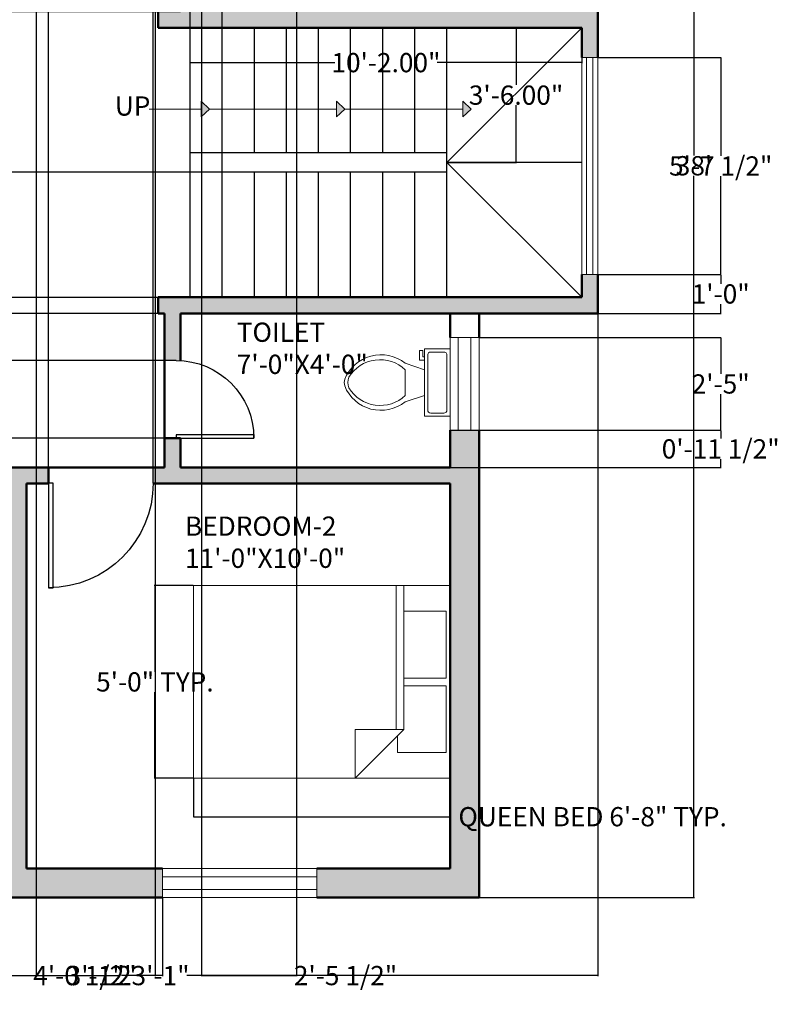
# Model space of a CAD drawing. Units: inches. Extents: x -19 to 356, y -14 to 509.
# Tile 2 of 3: x 118 to 355, y -14 to 293. Entities that reach past the tile are written whole.
import ezdxf

# ---------------------------------------------------------------- set-up
doc = ezdxf.new("R2010")
doc.units = ezdxf.units.IN
doc.header["$MEASUREMENT"] = 0
for name, color, linetype, lineweight in [('A-ANNO-DIMS', 7, 'Continuous', 18), ('A-ANNO-SYMB', 7, 'Continuous', 18), ('A-ANNO-TEXT', 7, 'Continuous', 18), ('A-AREA-IDEN', 7, 'Continuous', 25), ('A-DOOR', 3, 'Continuous', 25), ('A-FLOR-FIXT', 9, 'Continuous', 18), ('A-FLOR-STRS', 7, 'Continuous', 25), ('A-FURN', 8, 'Continuous', 18), ('A-GLAZ', 5, 'Continuous', 18), ('A-WALL', 7, 'Continuous', 50), ('A-WALL-PATT', 4, 'Continuous', 13)]:
    doc.layers.add(name, color=color, linetype=linetype, lineweight=lineweight)
doc.styles.get("Standard").update_dxf_attribs({"font": 'arial.ttf'})
doc.dimstyles.get("Standard").update_dxf_attribs({"dimtxt": 6, "dimasz": 0.18, "dimexe": 0.18, "dimexo": 0.0625, "dimgap": 0.09, "dimtad": 0, "dimtih": 1, "dimtoh": 1, "dimzin": 0, "dimdsep": 46, "dimlunit": 3, "dimtxsty": 'Standard', "dimcen": 0.09, "dimadec": 0, "dimazin": 0, "dimtfac": 1, "dimtofl": 0, "dimtmove": 0, "dimatfit": 3, "dimfxl": 1, "dimtolj": 1, "dimtzin": 0, "dimarcsym": 0})

# ---------------------------------------------------------------- blocks, each defined once
blk = doc.blocks.new('*U2')
for p, q in [((0, 0), (0, -6)), ((40, 0), (40, -6))]:
    blk.add_line(p, q)
blk.add_lwpolyline([(0, 0), (0, 40), (1.75, 40), (1.75, 0)], close=True)
blk.add_arc((0, 0), 40, 0, 90)
blk = doc.blocks.new('*U4')
for p, q in [((9.5, -6), (9.5, -2)), ((-10, -8.5), (-8, -8.5)), ((-10, -9.5), (-10, -8.5)), ((-8, -8.5), (-8, -8)), ((-7, -8), (-7, -9.5)), ((-4, -8), (-6, -14)), ((4, -8), (6, -14)), ((-7, -9.5), (-10, -9.5)), ((4, -14), (-4, -14))]:
    blk.add_line(p, q)
blk.add_lwpolyline([(10.5, -8), (10.5, 0), (-10.5, 0), (-10.5, -8)], close=True)
for points in [[(-9.5, -2), (-9.5, -6)], [(8.5, -1), (-8.5, -1)], [(-8.5, -7), (8.5, -7)]]:
    blk.add_lwpolyline(points)
for centre, radius, start, end in [((-8.62, -1.88), 0.884, 81.8699, 188.1301), ((8.62, -1.88), 0.884, 351.8699, 98.1301), ((-8.62, -6.12), 0.884, 171.8699, 278.1301), ((8.62, -6.12), 0.884, 261.8699, 8.1301), ((3.52, -21.58), 12.17, 141.4691, 247.9714), ((4.2, -21.82), 11.33, 136.3677, 238.9468), ((-3.52, -21.58), 12.17, 292.0284, 38.5307), ((-4.2, -21.82), 11.33, 301.053, 43.6321), ((0, -27.88), 4, 245.7318, 294.2682), ((0, -29), 4, 254.8605, 285.1395)]:
    blk.add_arc(centre, radius, start, end)
blk = doc.blocks.new('Bed - Queen')
for p, q in [((0, -80.00003), (0, 0)), ((0, 0), (59.99999, 0)), ((59.99999, 0), (59.99999, -80.00003)), ((7.99999, -1.2), (28.79998, -1.2)), ((7.99999, -14.4), (7.99999, -1.2)), ((28.79998, -1.2), (28.79998, -14.4)), ((31.19999, -1.2), (51.99999, -1.2)), ((31.19999, -14.4), (31.19999, -1.2)), ((51.99999, -1.2), (51.99999, -16.4)), ((0, -14.4), (44.8, -14.4)), ((59.99999, -29.6), (44.8, -14.4)), ((44.8, -14.4), (44.8, -29.6)), ((44.8, -16.8), (0, -16.8)), ((51.99999, -16.4), (46.79936, -16.4)), ((44.8, -29.6), (59.99999, -29.6)), ((59.99999, -80.00003), (0, -80.00003))]:
    blk.add_line(p, q)
blk = doc.blocks.new('*D8')
at = {"layer": 'A-ANNO-DIMS', "color": 0, "lineweight": -2, "transparency": 16777216}
for p, q in [((261.66, 475.37), (328.76, 475.37)), ((328.58, 475.19), (328.58, 250.53)), ((328.58, 19.55), (328.58, 244.22)), ((261.66, 19.37), (328.76, 19.37))]:
    blk.add_line(p, q, dxfattribs=at)
at = {"layer": 'A-ANNO-DIMS', "color": 0, "transparency": 16777216}
for points in [[(328.55, 475.19), (328.61, 475.19), (328.58, 475.37)], [(328.55, 19.55), (328.61, 19.55), (328.58, 19.37)]]:
    blk.add_solid(points, dxfattribs=at)
at = {"layer": 'Defpoints', "color": 0, "transparency": 16777216}
for p in [(261.6, 475.37), (328.58, 475.37), (261.6, 19.37)]:
    blk.add_point(p, dxfattribs=at)
at = {"layer": 'A-ANNO-DIMS', "color": 0, "transparency": 16777216, "insert": (328.58, 247.37), "char_height": 6, "attachment_point": 5}
blk.add_mtext("\\A1;38'", dxfattribs=at)
blk = doc.blocks.new('*D10')
at = {"layer": 'A-ANNO-DIMS', "color": 0, "lineweight": -2, "transparency": 16777216}
for p, q in [((171.6, 278.44), (171.6, 279.68)), ((171.78, 279.5), (216.66, 279.5)), ((293.42, 279.5), (248.54, 279.5)), ((293.6, 281.06), (293.6, 279.32))]:
    blk.add_line(p, q, dxfattribs=at)
at = {"layer": 'A-ANNO-DIMS', "color": 0, "transparency": 16777216}
for points in [[(171.78, 279.53), (171.78, 279.47), (171.6, 279.5)], [(293.42, 279.53), (293.42, 279.47), (293.6, 279.5)]]:
    blk.add_solid(points, dxfattribs=at)
at = {"layer": 'Defpoints', "color": 0, "transparency": 16777216}
for p in [(293.6, 281.12), (293.6, 279.5), (171.6, 278.38)]:
    blk.add_point(p, dxfattribs=at)
at = {"layer": 'A-ANNO-DIMS', "color": 0, "transparency": 16777216, "insert": (232.6, 279.5), "char_height": 6, "attachment_point": 5}
blk.add_mtext('\\A1;10\'-2.00"', dxfattribs=at)
blk = doc.blocks.new('*D11')
at = {"layer": 'A-ANNO-DIMS', "color": 0, "lineweight": -2, "transparency": 16777216}
for p, q in [((251.66, 290.37), (273.32, 290.37)), ((273.14, 290.19), (273.14, 272.53)), ((273.14, 248.55), (273.14, 266.22)), ((251.66, 248.37), (273.32, 248.37))]:
    blk.add_line(p, q, dxfattribs=at)
at = {"layer": 'A-ANNO-DIMS', "color": 0, "transparency": 16777216}
for points in [[(273.11, 290.19), (273.17, 290.19), (273.14, 290.37)], [(273.11, 248.55), (273.17, 248.55), (273.14, 248.37)]]:
    blk.add_solid(points, dxfattribs=at)
at = {"layer": 'Defpoints', "color": 0, "transparency": 16777216}
for p in [(251.6, 290.37), (273.14, 290.37), (251.6, 248.37)]:
    blk.add_point(p, dxfattribs=at)
at = {"layer": 'A-ANNO-DIMS', "color": 0, "transparency": 16777216, "insert": (273.14, 269.37), "char_height": 6, "attachment_point": 5}
blk.add_mtext('\\A1;3\'-6.00"', dxfattribs=at)
blk = doc.blocks.new('GLAZ-UNIT-48IN')
for p, q in [((0, 48), (0, 0)), ((4, 48), (4, 0))]:
    blk.add_line(p, q)
blk = doc.blocks.new('*D15')
at = {"layer": 'A-ANNO-DIMS', "color": 0, "lineweight": -2, "transparency": 16777216}
for p, q in [((172.6, 56.49), (172.6, 44.38)), ((252.6, 56.49), (252.6, 44.38)), ((172.78, 44.56), (252.42, 44.56)), ((252.6, 44.56), (252.78, 44.56))]:
    blk.add_line(p, q, dxfattribs=at)
at = {"layer": 'A-ANNO-DIMS', "color": 0, "transparency": 16777216}
for points in [[(172.78, 44.59), (172.78, 44.53), (172.6, 44.56)], [(252.42, 44.59), (252.42, 44.53), (252.6, 44.56)]]:
    blk.add_solid(points, dxfattribs=at)
at = {"layer": 'Defpoints', "color": 0, "transparency": 16777216}
for p in [(172.6, 56.56), (252.6, 56.56), (252.6, 44.56)]:
    blk.add_point(p, dxfattribs=at)
at = {"layer": 'A-ANNO-DIMS', "color": 0, "transparency": 16777216, "insert": (297, 44.56), "char_height": 6, "attachment_point": 5}
blk.add_mtext('\\A1;QUEEN BED 6\'-8" TYP.', dxfattribs=at)
blk = doc.blocks.new('*D16')
at = {"layer": 'A-ANNO-DIMS', "color": 0, "lineweight": -2, "transparency": 16777216}
for p, q in [((172.54, 116.56), (160.42, 116.56)), ((160.6, 116.38), (160.6, 89.71)), ((160.6, 56.74), (160.6, 83.4)), ((172.54, 56.56), (160.42, 56.56))]:
    blk.add_line(p, q, dxfattribs=at)
at = {"layer": 'A-ANNO-DIMS', "color": 0, "transparency": 16777216}
for points in [[(160.57, 116.38), (160.63, 116.38), (160.6, 116.56)], [(160.57, 56.74), (160.63, 56.74), (160.6, 56.56)]]:
    blk.add_solid(points, dxfattribs=at)
at = {"layer": 'Defpoints', "color": 0, "transparency": 16777216}
for p in [(172.6, 116.56), (160.6, 56.56), (172.6, 56.56)]:
    blk.add_point(p, dxfattribs=at)
at = {"layer": 'A-ANNO-DIMS', "color": 0, "transparency": 16777216, "insert": (160.6, 86.56), "char_height": 6, "attachment_point": 5}
blk.add_mtext('\\A1;5\'-0" TYP.', dxfattribs=at)
blk = doc.blocks.new('*D19')
at = {"layer": 'A-ANNO-DIMS', "color": 0, "lineweight": -2, "transparency": 16777216}
for p, q in [((298.6, 201.31), (298.6, -5.12)), ((21.6, 39.31), (21.6, -5.12)), ((21.78, -4.94), (149.65, -4.94)), ((298.42, -4.94), (170.55, -4.94))]:
    blk.add_line(p, q, dxfattribs=at)
at = {"layer": 'A-ANNO-DIMS', "color": 0, "transparency": 16777216}
for points in [[(21.78, -4.91), (21.78, -4.97), (21.6, -4.94)], [(298.42, -4.91), (298.42, -4.97), (298.6, -4.94)]]:
    blk.add_solid(points, dxfattribs=at)
at = {"layer": 'Defpoints', "color": 0, "transparency": 16777216}
for p in [(298.6, 201.37), (21.6, 39.37), (298.6, -4.94)]:
    blk.add_point(p, dxfattribs=at)
at = {"layer": 'A-ANNO-DIMS', "color": 0, "transparency": 16777216, "insert": (160.1, -4.94), "char_height": 6, "attachment_point": 5}
blk.add_mtext('\\A1;23\'-1"', dxfattribs=at)
blk = doc.blocks.new('*D29')
at = {"layer": 'A-ANNO-DIMS', "color": 0, "lineweight": -2, "transparency": 16777216}
for p, q in [((114.6, 19.31), (114.6, -5.12)), ((163.02, 19.31), (163.02, -5.12)), ((114.78, -4.94), (123.64, -4.94)), ((162.84, -4.94), (153.99, -4.94))]:
    blk.add_line(p, q, dxfattribs=at)
at = {"layer": 'A-ANNO-DIMS', "color": 0, "transparency": 16777216}
for points in [[(114.78, -4.91), (114.78, -4.97), (114.6, -4.94)], [(162.84, -4.91), (162.84, -4.97), (163.02, -4.94)]]:
    blk.add_solid(points, dxfattribs=at)
at = {"layer": 'Defpoints', "color": 0, "transparency": 16777216}
for p in [(114.6, 19.37), (163.02, 19.37), (114.6, -4.94)]:
    blk.add_point(p, dxfattribs=at)
at = {"layer": 'A-ANNO-DIMS', "color": 0, "transparency": 16777216, "insert": (138.81, -4.94), "char_height": 6, "attachment_point": 5}
blk.add_mtext('\\A1;4\'-0 1/2"', dxfattribs=at)
blk = doc.blocks.new('*D31')
at = {"layer": 'A-ANNO-DIMS', "color": 0, "lineweight": -2, "transparency": 16777216}
for p, q in [((123.6, 343.31), (123.6, -5.12)), ((160.72, 343.31), (160.72, -5.12)), ((123.78, -4.94), (134.1, -4.94)), ((160.54, -4.94), (150.22, -4.94))]:
    blk.add_line(p, q, dxfattribs=at)
at = {"layer": 'A-ANNO-DIMS', "color": 0, "transparency": 16777216}
for points in [[(123.78, -4.91), (123.78, -4.97), (123.6, -4.94)], [(160.54, -4.91), (160.54, -4.97), (160.72, -4.94)]]:
    blk.add_solid(points, dxfattribs=at)
at = {"layer": 'Defpoints', "color": 0, "transparency": 16777216}
for p in [(123.6, 343.37), (160.72, 343.37), (160.72, -4.94)]:
    blk.add_point(p, dxfattribs=at)
at = {"layer": 'A-ANNO-DIMS', "color": 0, "transparency": 16777216, "insert": (142.16, -4.94), "char_height": 6, "attachment_point": 5}
blk.add_mtext('\\A1;3\'-1"', dxfattribs=at)
blk = doc.blocks.new('*D32')
at = {"layer": 'A-ANNO-DIMS', "color": 0, "lineweight": -2, "transparency": 16777216}
for p, q in [((127.47, 153.44), (127.47, 499.87)), ((127.65, 499.69), (128.66, 499.69)), ((159.89, 499.69), (158.88, 499.69)), ((160.07, 153.44), (160.07, 499.87))]:
    blk.add_line(p, q, dxfattribs=at)
at = {"layer": 'A-ANNO-DIMS', "color": 0, "transparency": 16777216}
for points in [[(127.65, 499.72), (127.65, 499.66), (127.47, 499.69)], [(159.89, 499.72), (159.89, 499.66), (160.07, 499.69)]]:
    blk.add_solid(points, dxfattribs=at)
at = {"layer": 'Defpoints', "color": 0, "transparency": 16777216}
for p in [(160.07, 499.69), (127.47, 153.37), (160.07, 153.37)]:
    blk.add_point(p, dxfattribs=at)
at = {"layer": 'A-ANNO-DIMS', "color": 0, "transparency": 16777216, "insert": (143.77, 499.69), "char_height": 6, "attachment_point": 5}
blk.add_mtext('\\A1;2\'-8 1/2"', dxfattribs=at)
blk = doc.blocks.new('*D34')
at = {"layer": 'A-ANNO-DIMS', "color": 0, "lineweight": -2, "transparency": 16777216}
for p, q in [((175.13, 343.31), (175.13, -5.12)), ((204.73, 343.31), (204.73, -5.12)), ((175.31, -4.94), (204.55, -4.94)), ((204.73, -4.94), (204.91, -4.94))]:
    blk.add_line(p, q, dxfattribs=at)
at = {"layer": 'A-ANNO-DIMS', "color": 0, "transparency": 16777216}
for points in [[(175.31, -4.91), (175.31, -4.97), (175.13, -4.94)], [(204.55, -4.91), (204.55, -4.97), (204.73, -4.94)]]:
    blk.add_solid(points, dxfattribs=at)
at = {"layer": 'Defpoints', "color": 0, "transparency": 16777216}
for p in [(175.13, 343.37), (204.73, 343.37), (204.73, -4.94)]:
    blk.add_point(p, dxfattribs=at)
at = {"layer": 'A-ANNO-DIMS', "color": 0, "transparency": 16777216, "insert": (220.01, -4.94), "char_height": 6, "attachment_point": 5}
blk.add_mtext('\\A1;2\'-5 1/2"', dxfattribs=at)
blk = doc.blocks.new('*D35')
at = {"layer": 'A-ANNO-DIMS', "color": 0, "lineweight": -2, "transparency": 16777216}
for p, q in [((163.54, 186.72), (-2.9, 186.72)), ((-2.72, 186.54), (-2.72, 177.76)), ((-2.72, 162.67), (-2.72, 171.45)), ((163.54, 162.49), (-2.9, 162.49))]:
    blk.add_line(p, q, dxfattribs=at)
at = {"layer": 'A-ANNO-DIMS', "color": 0, "transparency": 16777216}
for points in [[(-2.75, 186.54), (-2.69, 186.54), (-2.72, 186.72)], [(-2.75, 162.67), (-2.69, 162.67), (-2.72, 162.49)]]:
    blk.add_solid(points, dxfattribs=at)
at = {"layer": 'Defpoints', "color": 0, "transparency": 16777216}
for p in [(-2.72, 186.72), (163.6, 186.72), (163.6, 162.49)]:
    blk.add_point(p, dxfattribs=at)
at = {"layer": 'A-ANNO-DIMS', "color": 0, "transparency": 16777216, "insert": (-2.72, 174.61), "char_height": 6, "attachment_point": 5}
blk.add_mtext('\\A1;2\'-0"', dxfattribs=at)
blk = doc.blocks.new('*D40')
at = {"layer": 'A-ANNO-DIMS', "color": 0, "lineweight": -2, "transparency": 16777216}
for p, q in [((168.54, 295.37), (-2.9, 295.37)), ((-2.72, 295.19), (-2.72, 251.53)), ((-2.72, 201.55), (-2.72, 245.22)), ((161.54, 201.37), (-2.9, 201.37))]:
    blk.add_line(p, q, dxfattribs=at)
at = {"layer": 'A-ANNO-DIMS', "color": 0, "transparency": 16777216}
for points in [[(-2.75, 295.19), (-2.69, 295.19), (-2.72, 295.37)], [(-2.75, 201.55), (-2.69, 201.55), (-2.72, 201.37)]]:
    blk.add_solid(points, dxfattribs=at)
at = {"layer": 'Defpoints', "color": 0, "transparency": 16777216}
for p in [(-2.72, 295.37), (168.6, 295.37), (161.6, 201.37)]:
    blk.add_point(p, dxfattribs=at)
at = {"layer": 'A-ANNO-DIMS', "color": 0, "transparency": 16777216, "insert": (-2.72, 248.37), "char_height": 6, "attachment_point": 5}
blk.add_mtext('\\A1;7\'-10"', dxfattribs=at)
blk = doc.blocks.new('*D41')
at = {"layer": 'A-ANNO-DIMS', "color": 0, "lineweight": -2, "transparency": 16777216}
for p, q in [((298.66, 281.12), (337.09, 281.12)), ((336.91, 280.94), (336.91, 250.49)), ((336.91, 213.66), (336.91, 244.11)), ((298.66, 213.48), (337.09, 213.48))]:
    blk.add_line(p, q, dxfattribs=at)
at = {"layer": 'A-ANNO-DIMS', "color": 0, "transparency": 16777216}
for points in [[(336.88, 280.94), (336.94, 280.94), (336.91, 281.12)], [(336.88, 213.66), (336.94, 213.66), (336.91, 213.48)]]:
    blk.add_solid(points, dxfattribs=at)
at = {"layer": 'Defpoints', "color": 0, "transparency": 16777216}
for p in [(298.6, 281.12), (336.91, 281.12), (298.6, 213.48)]:
    blk.add_point(p, dxfattribs=at)
at = {"layer": 'A-ANNO-DIMS', "color": 0, "transparency": 16777216, "insert": (336.91, 247.3), "char_height": 6, "attachment_point": 5}
blk.add_mtext('\\A1;5\'-7 1/2"', dxfattribs=at)
blk = doc.blocks.new('*D42')
at = {"layer": 'A-ANNO-DIMS', "color": 0, "lineweight": -2, "transparency": 16777216}
for p, q in [((261.66, 193.82), (337.09, 193.82)), ((336.91, 193.64), (336.91, 182.53)), ((336.91, 165.12), (336.91, 176.23)), ((261.66, 164.94), (337.09, 164.94))]:
    blk.add_line(p, q, dxfattribs=at)
at = {"layer": 'A-ANNO-DIMS', "color": 0, "transparency": 16777216}
for points in [[(336.88, 193.64), (336.94, 193.64), (336.91, 193.82)], [(336.88, 165.12), (336.94, 165.12), (336.91, 164.94)]]:
    blk.add_solid(points, dxfattribs=at)
at = {"layer": 'Defpoints', "color": 0, "transparency": 16777216}
for p in [(261.6, 193.82), (336.91, 193.82), (261.6, 164.94)]:
    blk.add_point(p, dxfattribs=at)
at = {"layer": 'A-ANNO-DIMS', "color": 0, "transparency": 16777216, "insert": (336.91, 179.38), "char_height": 6, "attachment_point": 5}
blk.add_mtext('\\A1;2\'-5"', dxfattribs=at)
blk = doc.blocks.new('*D43')
at = {"layer": 'A-ANNO-DIMS', "color": 0, "lineweight": -2, "transparency": 16777216}
for p, q in [((252.66, 164.94), (337.09, 164.94)), ((336.91, 164.76), (336.91, 162.35)), ((336.91, 153.55), (336.91, 155.96)), ((252.66, 153.37), (337.09, 153.37))]:
    blk.add_line(p, q, dxfattribs=at)
at = {"layer": 'A-ANNO-DIMS', "color": 0, "transparency": 16777216}
for points in [[(336.88, 164.76), (336.94, 164.76), (336.91, 164.94)], [(336.88, 153.55), (336.94, 153.55), (336.91, 153.37)]]:
    blk.add_solid(points, dxfattribs=at)
at = {"layer": 'Defpoints', "color": 0, "transparency": 16777216}
for p in [(252.6, 164.94), (336.91, 164.94), (252.6, 153.37)]:
    blk.add_point(p, dxfattribs=at)
at = {"layer": 'A-ANNO-DIMS', "color": 0, "transparency": 16777216, "insert": (336.91, 159.15), "char_height": 6, "attachment_point": 5}
blk.add_mtext('\\A1;0\'-11 1/2"', dxfattribs=at)
blk = doc.blocks.new('*D46')
at = {"layer": 'A-ANNO-DIMS', "color": 0, "lineweight": -2, "transparency": 16777216}
for p, q in [((298.66, 213.48), (337.09, 213.48)), ((336.91, 213.3), (336.91, 210.58)), ((336.91, 201.55), (336.91, 204.28)), ((298.66, 201.37), (337.09, 201.37))]:
    blk.add_line(p, q, dxfattribs=at)
at = {"layer": 'A-ANNO-DIMS', "color": 0, "transparency": 16777216}
for points in [[(336.88, 213.3), (336.94, 213.3), (336.91, 213.48)], [(336.88, 201.55), (336.94, 201.55), (336.91, 201.37)]]:
    blk.add_solid(points, dxfattribs=at)
at = {"layer": 'Defpoints', "color": 0, "transparency": 16777216}
for p in [(298.6, 213.48), (298.6, 201.37), (336.91, 201.37)]:
    blk.add_point(p, dxfattribs=at)
at = {"layer": 'A-ANNO-DIMS', "color": 0, "transparency": 16777216, "insert": (336.91, 207.43), "char_height": 6, "attachment_point": 5}
blk.add_mtext('\\A1;1\'-0"', dxfattribs=at)
blk = doc.blocks.new('*D47')
at = {"layer": 'A-ANNO-DIMS', "color": 0, "lineweight": -2, "transparency": 16777216}
for p, q in [((171.6, 206.44), (171.6, 499.87)), ((171.78, 499.69), (181.42, 499.69)), ((181.6, 206.44), (181.6, 499.87)), ((181.6, 499.69), (181.78, 499.69))]:
    blk.add_line(p, q, dxfattribs=at)
at = {"layer": 'A-ANNO-DIMS', "color": 0, "transparency": 16777216}
for points in [[(171.78, 499.72), (171.78, 499.66), (171.6, 499.69)], [(181.42, 499.72), (181.42, 499.66), (181.6, 499.69)]]:
    blk.add_solid(points, dxfattribs=at)
at = {"layer": 'Defpoints', "color": 0, "transparency": 16777216}
for p in [(181.6, 499.69), (171.6, 206.37), (181.6, 206.37)]:
    blk.add_point(p, dxfattribs=at)
at = {"layer": 'A-ANNO-DIMS', "color": 0, "transparency": 16777216, "insert": (192.18, 499.69), "char_height": 6, "attachment_point": 5}
blk.add_mtext('\\A1;0\'-10"', dxfattribs=at)
blk = doc.blocks.new('*D48')
at = {"layer": 'A-ANNO-DIMS', "color": 0, "lineweight": -2, "transparency": 16777216}
for p, q in [((171.54, 245.37), (-2.9, 245.37)), ((-2.72, 245.19), (-2.72, 229.03)), ((-2.72, 206.55), (-2.72, 222.72)), ((171.54, 206.37), (-2.9, 206.37))]:
    blk.add_line(p, q, dxfattribs=at)
at = {"layer": 'A-ANNO-DIMS', "color": 0, "transparency": 16777216}
for points in [[(-2.75, 245.19), (-2.69, 245.19), (-2.72, 245.37)], [(-2.75, 206.55), (-2.69, 206.55), (-2.72, 206.37)]]:
    blk.add_solid(points, dxfattribs=at)
at = {"layer": 'Defpoints', "color": 0, "transparency": 16777216}
for p in [(-2.72, 245.37), (171.6, 245.37), (171.6, 206.37)]:
    blk.add_point(p, dxfattribs=at)
at = {"layer": 'A-ANNO-DIMS', "color": 0, "transparency": 16777216, "insert": (-2.72, 225.87), "char_height": 6, "attachment_point": 5}
blk.add_mtext('\\A1;3\'-3"', dxfattribs=at)

msp = doc.modelspace()

# ---------------------------------------------------------------- hatches: boundary and pattern name
at = {"layer": 'A-ANNO-SYMB'}
h = msp.add_hatch(color=256, dxfattribs=at)
h.dxf.hatch_style = 1
h.paths.add_polyline_path([(256.554, 267.526), (256.554, 264.998), (256.554, 262.564), (259.193, 264.998)])
h.paths.add_polyline_path([(217.156, 267.526), (217.156, 264.998), (217.156, 262.564), (219.795, 264.998)])
h.paths.add_polyline_path([(175.002, 267.526), (175.002, 264.998), (175.002, 262.564), (177.641, 264.998)])
at = {"layer": 'A-WALL-PATT'}
h = msp.add_hatch(color=256, dxfattribs=at)
h.dxf.hatch_style = 1
h.paths.add_polyline_path([(30.6, 466.373), (88.282, 466.373), (88.282, 475.373), (21.6, 475.373), (21.6, 427.492), (30.6, 427.492)])
h.paths.add_polyline_path([(261.6, 475.373), (112.282, 475.373), (112.282, 466.373), (114.6, 466.373), (114.6, 349.373), (111.606, 349.373), (111.606, 348.938), (111.606, 343.373), (123.6, 343.373), (123.6, 349.373), (120.6, 349.373), (120.6, 466.373), (252.6, 466.373), (252.6, 424.113), (261.6, 424.113)])
h.paths.add_polyline_path([(261.6, 376.113), (252.6, 376.113), (252.6, 349.373), (204.767, 349.373), (204.767, 344.927, -0.0131156), (204.727, 343.373), (252.6, 343.373), (252.6, 335.439), (261.6, 335.439)])
h.paths.add_polyline_path([(261.6, 308.567), (252.6, 308.567), (252.6, 295.373), (261.6, 295.373)], flags=17)
h.paths.add_polyline_path([(298.6, 295.373), (168.6, 295.373), (168.6, 343.373), (175.128, 343.373), (175.128, 344.927), (175.128, 349.373), (160.722, 349.373, -0.0029301), (160.724, 348.938), (160.724, 343.373), (161.6, 343.373), (161.6, 290.373), (293.6, 290.373), (293.6, 281.12), (298.6, 281.12)])
h = msp.add_hatch(color=256, dxfattribs=at)
h.dxf.hatch_style = 1
h.paths.add_polyline_path([(74.504, 349.373), (30.6, 349.373), (30.6, 379.492), (21.6, 379.492), (21.6, 317.187), (30.6, 317.187), (30.6, 343.373), (74.504, 343.373)])
h.paths.add_polyline_path([(30.6, 269.187), (21.6, 269.187), (21.6, 235.01), (30.6, 235.01)])
h.paths.add_polyline_path([(30.6, 187.01), (21.6, 187.01), (21.6, 124.593), (30.6, 124.593), (30.6, 148.373), (74.604, 148.373), (74.604, 153.373), (30.6, 153.373)])
h.paths.add_polyline_path([(30.6, 76.593), (21.6, 76.593), (21.6, 39.373), (74.604, 39.373), (74.604, 44.312, -0.0309277), (74.855, 48.373), (30.6, 48.373)])
h.paths.add_polyline_path([(120.6, 148.373), (127.467, 148.373), (127.467, 148.483), (127.467, 153.373), (107.528, 153.373), (107.528, 148.373), (114.6, 148.373), (114.6, 19.373), (163.022, 19.373), (163.022, 28.373), (120.6, 28.373)])
h.paths.add_polyline_path([(114.6, 48.373), (107.528, 48.373), (107.528, 44.312), (107.528, 39.373), (114.6, 39.373)], flags=17)
h.paths.add_polyline_path([(261.6, 164.937), (252.6, 164.937), (252.6, 153.373), (168.6, 153.373), (168.6, 162.495), (167.233, 162.495), (163.6, 162.495), (163.6, 153.373), (160.071, 153.373), (160.071, 148.373), (252.6, 148.373), (252.6, 28.373), (211.022, 28.373), (211.022, 19.373), (261.6, 19.373)])
h.paths.add_polyline_path([(56.535, 228.167), (117.149, 228.167), (117.149, 250.555), (56.535, 250.555)], flags=9)
h.paths.add_polyline_path([(176.639, 359.092), (223.272, 359.092), (223.272, 381.481), (176.639, 381.481)], flags=9)
h = msp.add_hatch(color=256, dxfattribs=at)
h.dxf.hatch_style = 1
h.paths.add_polyline_path([(298.6, 213.484), (293.6, 213.484), (293.6, 206.373), (161.6, 206.373), (161.6, 201.373), (163.6, 201.373), (163.6, 186.717), (167.233, 186.717, -0.0141137), (168.6, 186.679), (168.6, 201.373), (261.6, 201.373), (298.6, 201.373)])

# ---------------------------------------------------------------- linework, layer by layer
at = {"layer": 'A-ANNO-SYMB'}
for p, q in [((171.6, 264.998), (158.782, 264.998)), ((158.782, 264.998), (175.002, 264.998)), ((171.6, 264.998), (175.002, 264.998)), ((177.641, 264.998), (217.156, 264.998)), ((219.795, 264.998), (256.554, 264.998))]:
    msp.add_line(p, q, dxfattribs=at)
for points in [[(175.002, 264.998), (175.002, 262.564), (177.641, 264.998), (175.002, 267.526)], [(217.156, 264.998), (217.156, 262.564), (219.795, 264.998), (217.156, 267.526)], [(256.554, 264.998), (256.554, 262.564), (259.193, 264.998), (256.554, 267.526)]]:
    msp.add_lwpolyline(points, close=True, dxfattribs=at)
at = {"layer": 'A-FLOR-FIXT'}
msp.add_lwpolyline([(252.6, 169.318), (252.6, 190.318)], dxfattribs=at)
at = {"layer": 'A-FLOR-STRS'}
for p, q in [((251.6, 248.373), (293.6, 290.373)), ((251.6, 251.373), (171.6, 251.373)), ((293.6, 248.373), (251.6, 248.373)), ((251.6, 248.373), (293.6, 206.373)), ((251.6, 245.373), (171.6, 245.373))]:
    msp.add_line(p, q, dxfattribs=at)
for points in [[(171.6, 206.373), (171.6, 290.373)], [(181.6, 251.373), (181.6, 290.373)], [(191.6, 251.373), (191.6, 290.373)], [(201.6, 251.373), (201.6, 290.373)], [(211.6, 251.373), (211.6, 290.373)], [(221.6, 251.373), (221.6, 290.373)], [(231.6, 251.373), (231.6, 290.373)], [(241.6, 251.373), (241.6, 290.373)], [(251.6, 206.373), (251.6, 290.373)], [(181.6, 206.373), (181.6, 245.373)], [(191.6, 206.373), (191.6, 245.373)], [(201.6, 206.373), (201.6, 245.373)], [(211.6, 206.373), (211.6, 245.373)], [(221.6, 206.373), (221.6, 245.373)], [(231.6, 206.373), (231.6, 245.373)], [(241.6, 206.373), (241.6, 245.373)]]:
    msp.add_lwpolyline(points, dxfattribs=at)
at = {"layer": 'A-GLAZ'}
for p, q in [((295.1, 281.12), (295.1, 213.484)), ((297.1, 281.12), (297.1, 213.484)), ((255.1, 164.937), (255.1, 193.82)), ((259.1, 164.937), (259.1, 193.82))]:
    msp.add_line(p, q, dxfattribs=at)
for points in [[(293.6, 213.484), (298.6, 213.484), (298.6, 281.12), (293.6, 281.12)], [(252.6, 193.82), (261.6, 193.82), (261.6, 164.937), (252.6, 164.937)], [(163.022, 28.373), (211.022, 28.373), (211.022, 19.373), (163.022, 19.373)]]:
    msp.add_lwpolyline(points, close=True, dxfattribs=at)
at = {"layer": 'A-WALL'}
for p, q in [((163.6, 162.495), (168.6, 162.495)), ((127.467, 148.373), (127.467, 153.373))]:
    msp.add_line(p, q, dxfattribs=at)
for points in [[(161.6, 290.373), (161.6, 343.373)], [(298.6, 281.12), (298.6, 295.373)], [(293.6, 290.373), (161.6, 290.373)], [(293.6, 281.12), (293.6, 290.373)], [(293.6, 206.373), (293.6, 213.484)], [(298.6, 201.373), (298.6, 213.484)], [(293.6, 206.373), (161.6, 206.373)], [(161.6, 201.373), (161.6, 206.373)], [(163.6, 201.373), (161.6, 201.373)], [(163.6, 153.373), (163.6, 201.373)], [(261.6, 201.373), (168.6, 201.373)], [(298.6, 201.373), (168.6, 201.373)], [(168.6, 186.679), (168.6, 201.373)], [(252.6, 193.82), (252.6, 201.373)], [(261.6, 193.82), (261.6, 201.373)], [(211.022, 19.373), (261.6, 19.373), (261.6, 164.937)], [(252.6, 153.373), (252.6, 164.937)], [(168.6, 153.373), (168.6, 162.495)], [(163.6, 153.373), (30.6, 153.373)], [(252.6, 153.373), (168.6, 153.373)], [(120.6, 28.373), (120.6, 148.373)], [(127.487, 148.373), (120.6, 148.373)], [(252.6, 148.373), (160.091, 148.373)], [(252.6, 28.373), (252.6, 148.373)], [(120.6, 28.373), (163.022, 28.373)], [(211.022, 28.373), (252.6, 28.373)], [(114.6, 19.373), (163.022, 19.373)]]:
    msp.add_lwpolyline(points, dxfattribs=at)

# ---------------------------------------------------------------- block references
at = {"layer": 'A-DOOR'}
for p, xscale, yscale, zscale, rotation in [((167.233, 162.495), -0.605558797889584, 0.605558797889584, 0.605558797889584, 270), ((127.467, 148.483), -0.8150853580163643, 0.8150853580163643, 0.8150853580163643, 180)]:
    msp.add_blockref('*U2', p, dxfattribs=dict(at, xscale=xscale, yscale=yscale, zscale=zscale, rotation=rotation))
at = {"layer": 'A-FLOR-FIXT', "rotation": 270}
msp.add_blockref('*U4', (252.6, 179.818), dxfattribs=at)
at = {"layer": 'A-FURN', "rotation": 270}
msp.add_blockref('Bed - Queen', (252.6, 116.557), dxfattribs=at)
at = {"layer": 'A-GLAZ', "rotation": 269.9999999999999}
msp.add_blockref('GLAZ-UNIT-48IN', (163.022, 25.873), dxfattribs=at)

# ---------------------------------------------------------------- texts
at = {"layer": 'A-ANNO-TEXT', "insert": (138.957, 268.989), "char_height": 6, "attachment_point": 1}
msp.add_mtext_dynamic_manual_height_columns('     UP', width=102.62239, gutter_width=1, heights=[0], dxfattribs=at)
at = {"layer": 'A-AREA-IDEN', "char_height": 6, "attachment_point": 1}
for s, insert in [('TOILET\\P7\'-0"X4\'-0"', (186.11, 198.506)), ('BEDROOM-2\\P11\'-0"X10\'-0"', (169.978, 138.086))]:
    msp.add_mtext_dynamic_manual_height_columns(s, width=23.41838, gutter_width=1, heights=[0], dxfattribs=dict(at, insert=insert))

# ---------------------------------------------------------------- dimensions: what is measured, and where the dimension line sits
at = {"layer": 'A-ANNO-DIMS'}
for base, p1, p2, override, picture, middle in [((160.071, 499.688), (127.467, 153.373), (160.071, 153.373), {"dimdec": 1, "dimlfac": 1, "dimrnd": 0, "dimzin": 1, "dimdsep": 46, "dimlunit": 4, "dimfrac": 2}, '*D32', (143.769, 499.688)), ((181.6, 499.688), (171.6, 206.373), (181.6, 206.373), {"dimdec": 1, "dimlfac": 1, "dimrnd": 0, "dimzin": 1, "dimdsep": 46, "dimlunit": 4, "dimfrac": 2}, '*D47', (192.176, 499.688)), ((160.724, -4.942), (123.6, 343.373), (160.724, 343.373), {"dimdec": 1, "dimlfac": 1, "dimrnd": 0, "dimzin": 1, "dimdsep": 46, "dimlunit": 4, "dimfrac": 2}, '*D31', (142.162, -4.942)), ((204.727, -4.942), (175.128, 343.373), (204.727, 343.373), {"dimdec": 1, "dimlfac": 1, "dimrnd": 0, "dimzin": 1, "dimdsep": 46, "dimlunit": 4, "dimfrac": 2}, '*D34', (220.013, -4.942)), ((293.6, 279.501), (171.6, 278.381), (293.6, 281.12), {"dimclrd": 0, "dimclre": 0, "dimclrt": 0}, '*D10', (232.6, 279.501)), ((298.6, -4.942), (21.6, 39.373), (298.6, 201.373), {"dimdec": 1, "dimlfac": 1, "dimrnd": 0, "dimzin": 1, "dimdsep": 46, "dimlunit": 4, "dimfrac": 2}, '*D19', (160.1, -4.942)), ((114.6, -4.942), (163.022, 19.373), (114.6, 19.373), {"dimdec": 1, "dimlfac": 1, "dimrnd": 0, "dimzin": 1, "dimdsep": 46, "dimlunit": 4, "dimfrac": 2}, '*D29', (138.811, -4.942))]:
    dim = msp.add_linear_dim(base=base, p1=p1, p2=p2, dimstyle='Standard', override=override, dxfattribs=at)
    dim.commit()
    dim.dimension.update_dxf_attribs({"geometry": picture, "text_midpoint": middle})
for base, p1, p2, override, picture, middle in [((328.581, 475.373), (261.6, 19.373), (261.6, 475.373), {"dimclrd": 0, "dimclre": 0, "dimclrt": 0}, '*D8', (328.581, 247.373)), ((-2.715, 295.373), (161.6, 201.373), (168.6, 295.373), {"dimdec": 1, "dimlfac": 1, "dimrnd": 0, "dimzin": 1, "dimdsep": 46, "dimlunit": 4, "dimfrac": 2}, '*D40', (-2.715, 248.373)), ((273.142, 290.373), (251.6, 248.373), (251.6, 290.373), {"dimclrd": 0, "dimclre": 0, "dimclrt": 0}, '*D11', (273.142, 269.373)), ((336.915, 281.12), (298.6, 213.484), (298.6, 281.12), {"dimdec": 1, "dimlfac": 1, "dimrnd": 0, "dimzin": 1, "dimdsep": 46, "dimlunit": 4, "dimfrac": 2}, '*D41', (336.915, 247.302)), ((-2.715, 245.373), (171.6, 206.373), (171.6, 245.373), {"dimdec": 1, "dimlfac": 1, "dimrnd": 0, "dimzin": 1, "dimdsep": 46, "dimlunit": 4, "dimfrac": 2}, '*D48', (-2.715, 225.873)), ((336.915, 201.373), (298.6, 213.484), (298.6, 201.373), {"dimdec": 1, "dimlfac": 1, "dimrnd": 0, "dimzin": 1, "dimdsep": 46, "dimlunit": 4, "dimfrac": 2}, '*D46', (336.915, 207.429)), ((336.915, 193.82), (261.6, 164.937), (261.6, 193.82), {"dimdec": 1, "dimlfac": 1, "dimrnd": 0, "dimzin": 1, "dimdsep": 46, "dimlunit": 4, "dimfrac": 2}, '*D42', (336.915, 179.378)), ((-2.715, 186.717), (163.6, 162.495), (163.6, 186.717), {"dimdec": 1, "dimlfac": 1, "dimrnd": 0, "dimzin": 1, "dimdsep": 46, "dimlunit": 4, "dimfrac": 2}, '*D35', (-2.715, 174.606)), ((336.915, 164.937), (252.6, 153.373), (252.6, 164.937), {"dimdec": 1, "dimlfac": 1, "dimrnd": 0, "dimzin": 1, "dimdsep": 46, "dimlunit": 4, "dimfrac": 2}, '*D43', (336.915, 159.155))]:
    dim = msp.add_linear_dim(base=base, p1=p1, p2=p2, angle=90, dimstyle='Standard', override=override, dxfattribs=at)
    dim.commit()
    dim.dimension.update_dxf_attribs({"geometry": picture, "text_midpoint": middle})
dim = msp.add_linear_dim(base=(160.6, 56.557), p1=(172.6, 116.557), p2=(172.6, 56.557), angle=270, text='<> TYP.', dimstyle='Standard', override={"dimdec": 1, "dimlfac": 1, "dimrnd": 0, "dimzin": 1, "dimdsep": 46, "dimlunit": 4, "dimfrac": 2}, dxfattribs=at)
dim.commit()
dim.dimension.update_dxf_attribs({"geometry": '*D16', "text_midpoint": (160.6, 86.557)})
dim = msp.add_linear_dim(base=(252.6, 44.557), p1=(172.6, 56.557), p2=(252.6, 56.557), text='QUEEN BED <> TYP.', dimstyle='Standard', override={"dimdec": 1, "dimlfac": 1, "dimrnd": 0, "dimzin": 1, "dimdsep": 46, "dimlunit": 4, "dimfrac": 2}, dxfattribs=at)
dim.commit()
dim.dimension.update_dxf_attribs({"geometry": '*D15', "text_midpoint": (297, 44.557)})

doc.saveas('drawing.dxf')
